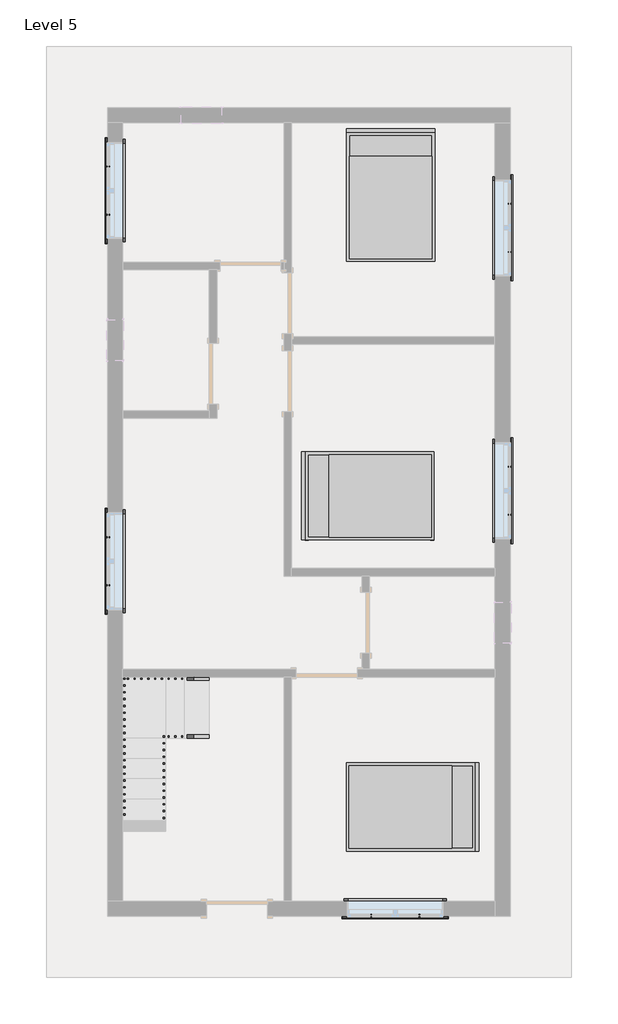
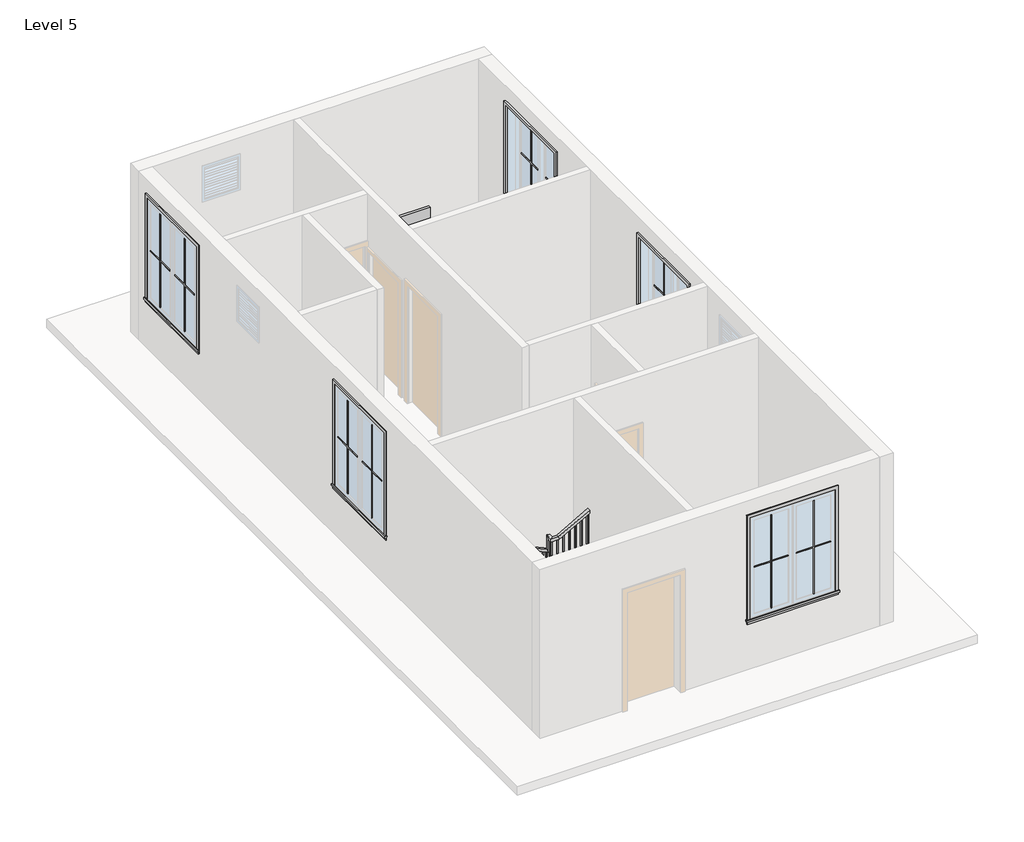
# One storey, part 2 of 2: 20 proxies, 3 furniture elements, 2 railings.
"""IFC4 building model written with IfcOpenShell, lengths in millimetres."""

from ifc_helpers import new_model, si_unit, frame, origin, place, context, project, spatial, polyline, outline, extrude, faceted_brep, transform, mapped, element, save
from components import muntin_pattern_2x2_muntin_pattern_2x2_bff912c5, muntin_pattern_2x2_muntin_pattern_2x2_c2194282, trim_window_exterior_flat_with_sill_e04b3088, trim_window_interior_flat_picture_frame_2a7685fe, bed_17739_bed_17739_15c61121

model = new_model("IFC4")

# Units and contexts
model_context = context("Model", 3, world=origin())
ifc_project = project(units=[si_unit("LENGTHUNIT", "METRE", prefix="MILLI")], contexts=[model_context])

# Site, building, storey
site = spatial("IfcSite", under=ifc_project)
building = spatial("IfcBuilding", under=site)
storey = spatial("IfcBuildingStorey", under=building, Name="Level 5", Elevation=9601.2)

# Proxies
placement = place(None, origin())
muntin_pattern_2x2_muntin_pattern_2x2_shape = muntin_pattern_2x2_muntin_pattern_2x2_bff912c5(model_context)
element("IfcBuildingElementProxy", 1, Name="Muntin Pattern_2x2 : Muntin Pattern_2x2", ObjectType="Muntin Pattern_2x2 : Muntin Pattern_2x2", at=placement, inside=storey, context=model_context, shape_type="MappedRepresentation", body=[
    mapped(muntin_pattern_2x2_muntin_pattern_2x2_shape, transform((-4261.9639285, 4584.2694249, 10585.45), x_axis=(0.0, 1.0, 0.0), y_axis=(-1.0, 0.0, 0.0), z_axis=(0.0, 0.0, 1.0))),
])
element("IfcBuildingElementProxy", 2, Name="Muntin Pattern_2x2 : Muntin Pattern_2x2", ObjectType="Muntin Pattern_2x2 : Muntin Pattern_2x2", at=placement, inside=storey, context=model_context, shape_type="MappedRepresentation", body=[
    mapped(muntin_pattern_2x2_muntin_pattern_2x2_shape, transform((1751.4860715, 4746.1944249, 10585.45), x_axis=(0.0, -1.0, 0.0), y_axis=(1.0, 0.0, 0.0), z_axis=(0.0, 0.0, 1.0))),
])
element("IfcBuildingElementProxy", 3, Name="Muntin Pattern_2x2 : Muntin Pattern_2x2", ObjectType="Muntin Pattern_2x2 : Muntin Pattern_2x2", at=placement, inside=storey, context=model_context, shape_type="MappedRepresentation", body=[
    mapped(muntin_pattern_2x2_muntin_pattern_2x2_shape, transform((-4261.9639285, -962.4555751, 10585.45), x_axis=(0.0, 1.0, 0.0), y_axis=(-1.0, 0.0, 0.0), z_axis=(0.0, 0.0, 1.0))),
])
element("IfcBuildingElementProxy", 4, Name="Muntin Pattern_2x2 : Muntin Pattern_2x2", ObjectType="Muntin Pattern_2x2 : Muntin Pattern_2x2", at=placement, inside=storey, context=model_context, shape_type="MappedRepresentation", body=[
    mapped(muntin_pattern_2x2_muntin_pattern_2x2_shape, transform((1751.4860715, 812.3694249, 10585.45), x_axis=(0.0, -1.0, 0.0), y_axis=(1.0, 0.0, 0.0), z_axis=(0.0, 0.0, 1.0))),
])
element("IfcBuildingElementProxy", 5, Name="Muntin Pattern_2x2 : Muntin Pattern_2x2", ObjectType="Muntin Pattern_2x2 : Muntin Pattern_2x2", at=placement, inside=storey, context=model_context, shape_type="MappedRepresentation", body=[
    mapped(muntin_pattern_2x2_muntin_pattern_2x2_shape, transform((397.3485715, -5907.5180751, 10585.45), x_axis=(-1.0, 0.0, 0.0), y_axis=(0.0, -1.0, 0.0), z_axis=(0.0, 0.0, 1.0))),
])
muntin_pattern_2x2_muntin_pattern_2x2_2_shape = muntin_pattern_2x2_muntin_pattern_2x2_c2194282(model_context)
element("IfcBuildingElementProxy", 6, Name="Muntin Pattern_2x2 : Muntin Pattern_2x2", ObjectType="Muntin Pattern_2x2 : Muntin Pattern_2x2", at=placement, inside=storey, context=model_context, shape_type="MappedRepresentation", body=[
    mapped(muntin_pattern_2x2_muntin_pattern_2x2_2_shape, transform((-4261.9639285, 5304.9944249, 10585.45), x_axis=(0.0, -1.0, 0.0), y_axis=(1.0, 0.0, 0.0), z_axis=(0.0, 0.0, 1.0))),
])
element("IfcBuildingElementProxy", 7, Name="Muntin Pattern_2x2 : Muntin Pattern_2x2", ObjectType="Muntin Pattern_2x2 : Muntin Pattern_2x2", at=placement, inside=storey, context=model_context, shape_type="MappedRepresentation", body=[
    mapped(muntin_pattern_2x2_muntin_pattern_2x2_2_shape, transform((1751.4860715, 4025.4694249, 10585.45), x_axis=(0.0, 1.0, 0.0), y_axis=(-1.0, 0.0, 0.0), z_axis=(0.0, 0.0, 1.0))),
])
element("IfcBuildingElementProxy", 8, Name="Muntin Pattern_2x2 : Muntin Pattern_2x2", ObjectType="Muntin Pattern_2x2 : Muntin Pattern_2x2", at=placement, inside=storey, context=model_context, shape_type="MappedRepresentation", body=[
    mapped(muntin_pattern_2x2_muntin_pattern_2x2_2_shape, transform((-4261.9639285, -241.7305751, 10585.45), x_axis=(0.0, -1.0, 0.0), y_axis=(1.0, 0.0, 0.0), z_axis=(0.0, 0.0, 1.0))),
])
element("IfcBuildingElementProxy", 9, Name="Muntin Pattern_2x2 : Muntin Pattern_2x2", ObjectType="Muntin Pattern_2x2 : Muntin Pattern_2x2", at=placement, inside=storey, context=model_context, shape_type="MappedRepresentation", body=[
    mapped(muntin_pattern_2x2_muntin_pattern_2x2_2_shape, transform((1751.4860715, 91.6444249, 10585.45), x_axis=(0.0, 1.0, 0.0), y_axis=(-1.0, 0.0, 0.0), z_axis=(0.0, 0.0, 1.0))),
])
element("IfcBuildingElementProxy", 10, Name="Muntin Pattern_2x2 : Muntin Pattern_2x2", ObjectType="Muntin Pattern_2x2 : Muntin Pattern_2x2", at=placement, inside=storey, context=model_context, shape_type="MappedRepresentation", body=[
    mapped(muntin_pattern_2x2_muntin_pattern_2x2_2_shape, transform((-323.3764285, -5907.5180751, 10585.45), x_axis=(1.0, 0.0, 0.0), y_axis=(0.0, 1.0, 0.0), z_axis=(0.0, 0.0, 1.0))),
])
trim_window_exterior_flat_with_sill_shape = trim_window_exterior_flat_with_sill_e04b3088(model_context)
element("IfcBuildingElementProxy", 11, Name="Trim-Window-Exterior-Flat : with Sill", ObjectType="Trim-Window-Exterior-Flat : with Sill", at=placement, inside=storey, context=model_context, shape_type="MappedRepresentation", body=[
    mapped(trim_window_exterior_flat_with_sill_shape, transform((-4271.4889285, 4944.6319249, 12344.4), x_axis=(0.0, -1.0, 0.0), y_axis=(0.0, 0.0, 1.0), z_axis=(-1.0, 0.0, 0.0))),
])
element("IfcBuildingElementProxy", 12, Name="Trim-Window-Exterior-Flat : with Sill", ObjectType="Trim-Window-Exterior-Flat : with Sill", at=placement, inside=storey, context=model_context, shape_type="MappedRepresentation", body=[
    mapped(trim_window_exterior_flat_with_sill_shape, transform((1761.0110715, 4385.8319249, 12344.4), x_axis=(0.0, 1.0, 0.0), y_axis=(0.0, 0.0, 1.0), z_axis=(1.0, 0.0, 0.0))),
])
element("IfcBuildingElementProxy", 13, Name="Trim-Window-Exterior-Flat : with Sill", ObjectType="Trim-Window-Exterior-Flat : with Sill", at=placement, inside=storey, context=model_context, shape_type="MappedRepresentation", body=[
    mapped(trim_window_exterior_flat_with_sill_shape, transform((-4271.4889285, -602.0930751, 12344.4), x_axis=(0.0, -1.0, 0.0), y_axis=(0.0, 0.0, 1.0), z_axis=(-1.0, 0.0, 0.0))),
])
element("IfcBuildingElementProxy", 14, Name="Trim-Window-Exterior-Flat : with Sill", ObjectType="Trim-Window-Exterior-Flat : with Sill", at=placement, inside=storey, context=model_context, shape_type="MappedRepresentation", body=[
    mapped(trim_window_exterior_flat_with_sill_shape, transform((1761.0110715, 452.0069249, 12344.4), x_axis=(0.0, 1.0, 0.0), y_axis=(0.0, 0.0, 1.0), z_axis=(1.0, 0.0, 0.0))),
])
element("IfcBuildingElementProxy", 15, Name="Trim-Window-Exterior-Flat : with Sill", ObjectType="Trim-Window-Exterior-Flat : with Sill", at=placement, inside=storey, context=model_context, shape_type="MappedRepresentation", body=[
    mapped(trim_window_exterior_flat_with_sill_shape, transform((36.9860715, -5917.0430751, 12344.4), x_axis=(1.0, 0.0, 0.0), y_axis=(0.0, 0.0, 1.0), z_axis=(0.0, -1.0, 0.0))),
])
trim_window_interior_flat_picture_frame_shape = trim_window_interior_flat_picture_frame_2a7685fe(model_context)
element("IfcBuildingElementProxy", 16, Name="Trim-Window-Interior-Flat : Picture Frame", ObjectType="Trim-Window-Interior-Flat : Picture Frame", at=placement, inside=storey, context=model_context, shape_type="MappedRepresentation", body=[
    mapped(trim_window_interior_flat_picture_frame_shape, transform((-4042.8889285, 4944.6319249, 12344.4), x_axis=(0.0, 1.0, 0.0), y_axis=(0.0, 0.0, 1.0), z_axis=(1.0, 0.0, 0.0))),
])
element("IfcBuildingElementProxy", 17, Name="Trim-Window-Interior-Flat : Picture Frame", ObjectType="Trim-Window-Interior-Flat : Picture Frame", at=placement, inside=storey, context=model_context, shape_type="MappedRepresentation", body=[
    mapped(trim_window_interior_flat_picture_frame_shape, transform((1532.4110715, 4385.8319249, 12344.4), x_axis=(0.0, -1.0, 0.0), y_axis=(0.0, 0.0, 1.0), z_axis=(-1.0, 0.0, 0.0))),
])
element("IfcBuildingElementProxy", 18, Name="Trim-Window-Interior-Flat : Picture Frame", ObjectType="Trim-Window-Interior-Flat : Picture Frame", at=placement, inside=storey, context=model_context, shape_type="MappedRepresentation", body=[
    mapped(trim_window_interior_flat_picture_frame_shape, transform((-4042.8889285, -602.0930751, 12344.4), x_axis=(0.0, 1.0, 0.0), y_axis=(0.0, 0.0, 1.0), z_axis=(1.0, 0.0, 0.0))),
])
element("IfcBuildingElementProxy", 19, Name="Trim-Window-Interior-Flat : Picture Frame", ObjectType="Trim-Window-Interior-Flat : Picture Frame", at=placement, inside=storey, context=model_context, shape_type="MappedRepresentation", body=[
    mapped(trim_window_interior_flat_picture_frame_shape, transform((1532.4110715, 452.0069249, 12344.4), x_axis=(0.0, -1.0, 0.0), y_axis=(0.0, 0.0, 1.0), z_axis=(-1.0, 0.0, 0.0))),
])
element("IfcBuildingElementProxy", 20, Name="Trim-Window-Interior-Flat : Picture Frame", ObjectType="Trim-Window-Interior-Flat : Picture Frame", at=placement, inside=storey, context=model_context, shape_type="MappedRepresentation", body=[
    mapped(trim_window_interior_flat_picture_frame_shape, transform((36.9860715, -5688.4430751, 12344.4), x_axis=(-1.0, 0.0, 0.0), y_axis=(0.0, 0.0, 1.0), z_axis=(0.0, 1.0, 0.0))),
])

# Furniture
bed_17739_bed_17739_shape = bed_17739_bed_17739_15c61121(model_context)
element("IfcFurniture", 21, ObjectType="Bed_17739 : Bed_17739", at=placement, inside=storey, context=model_context, shape_type="MappedRepresentation", body=[
    mapped(bed_17739_bed_17739_shape, transform((-29.6889285, 4852.5569249, 9601.2), x_axis=(1.0, 0.0, 0.0), y_axis=(0.0, 1.0, 0.0), z_axis=(0.0, 0.0, 1.0))),
])
element("IfcFurniture", 22, ObjectType="Bed_17739 : Bed_17739", at=placement, inside=storey, context=model_context, shape_type="MappedRepresentation", body=[
    mapped(bed_17739_bed_17739_shape, transform((-347.1889285, 375.8069249, 9601.2), x_axis=(0.0, 1.0, 0.0), y_axis=(-1.0, 0.0, 0.0), z_axis=(0.0, 0.0, 1.0))),
])
element("IfcFurniture", 23, ObjectType="Bed_17739 : Bed_17739", at=placement, inside=storey, context=model_context, shape_type="MappedRepresentation", body=[
    mapped(bed_17739_bed_17739_shape, transform((275.1110715, -4278.7430751, 9601.2), x_axis=(0.0, -1.0, 0.0), y_axis=(1.0, 0.0, 0.0), z_axis=(0.0, 0.0, 1.0))),
])

# Railings
element("IfcRailing", 24, ObjectType="Handrail - Rectangular", at=placement, inside=storey, context=model_context, shape_type="SolidModel", body=[
    faceted_brep([(-2747.4889285, -2386.4430751, 10684.9333333), (-2747.4889285, -2386.4430751, 10627.7271159), (-2747.4889285, -2335.6430751, 10627.7271159), (-2747.4889285, -2335.6430751, 10684.9333333), (-3396.0267484, -2386.4430751, 11020.7457967), (-3408.3987558, -2386.4430751, 10969.9457967), (-3408.3987558, -2335.6430751, 10969.9457967), (-3396.0267484, -2335.6430751, 11020.7457967), (-3992.0889285, -2386.4430751, 11020.7457967), (-3992.0889285, -2386.4430751, 10969.9457967), (-4042.8889285, -2335.6430751, 10969.9457967), (-4042.8889285, -2335.6430751, 11020.7457967), (-3992.0889285, -2940.1628326, 11020.7457967), (-3992.0889285, -2953.3285634, 10969.9457967), (-4042.8889285, -2953.3285634, 10969.9457967), (-4042.8889285, -2940.1628326, 11020.7457967), (-3992.0889285, -5061.9991591, 12199.7618165), (-3992.0889285, -5075.1648899, 12148.9618165), (-4042.8889285, -5075.1648899, 12148.9618165), (-4042.8889285, -5061.9991591, 12199.7618165), (-3992.0889285, -5637.6430751, 12199.7618165), (-3992.0889285, -5637.6430751, 12148.9618165), (-4042.8889285, -5688.4430751, 12148.9618165), (-4042.8889285, -5688.4430751, 12199.7618165), (-3418.001852, -5637.6430751, 12199.7618165), (-3404.8062484, -5637.6430751, 12148.9618165), (-3404.8062484, -5688.4430751, 12148.9618165), (-3418.001852, -5688.4430751, 12199.7618165), (-2793.6303845, -5637.6430751, 12547.6), (-2793.6303845, -5688.4430751, 12547.6), (-2793.6303845, -5688.4430751, 12489.4487115), (-2793.6303845, -5637.6430751, 12489.4487115)], [[[0, 1, 2, 3]], [[1, 0, 4, 5]], [[2, 1, 5, 6]], [[3, 2, 6, 7]], [[0, 3, 7, 4]], [[5, 4, 8, 9]], [[6, 5, 9, 10]], [[7, 6, 10, 11]], [[4, 7, 11, 8]], [[9, 8, 12, 13]], [[10, 9, 13, 14]], [[11, 10, 14, 15]], [[8, 11, 15, 12]], [[13, 12, 16, 17]], [[14, 13, 17, 18]], [[15, 14, 18, 19]], [[12, 15, 19, 16]], [[17, 16, 20, 21]], [[18, 17, 21, 22]], [[19, 18, 22, 23]], [[16, 19, 23, 20]], [[21, 20, 24, 25]], [[22, 21, 25, 26]], [[23, 22, 26, 27]], [[20, 23, 27, 24]], [[28, 29, 30, 31]], [[25, 24, 28, 31]], [[26, 25, 31, 30]], [[27, 26, 30, 29]], [[24, 27, 29, 28]]]),
    extrude(outline(polyline([(12492.1598207, -2788.7639285), (12481.5470401, -2807.8139285), (11463.8666667, -2807.8139285), (11463.8666667, -2788.7639285), (12492.1598207, -2788.7639285)])), frame((0.0, -5672.5680751, 0.0), z_axis=(0.0, 1.0, 0.0), x_axis=(0.0, 0.0, 1.0)), (0.0, 0.0, 1.0), 19.05),
    extrude(outline(polyline([(12435.5583242, -2890.3639285), (12424.9455436, -2909.4139285), (11463.8666667, -2909.4139285), (11463.8666667, -2890.3639285), (12435.5583242, -2890.3639285)])), frame((0.0, -5672.5680751, 0.0), z_axis=(0.0, 1.0, 0.0), x_axis=(0.0, 0.0, 1.0)), (0.0, 0.0, 1.0), 19.05),
    extrude(outline(polyline([(12378.9568277, -2991.9639285), (12368.3440471, -3011.0139285), (11463.8666667, -3011.0139285), (11463.8666667, -2991.9639285), (12378.9568277, -2991.9639285)])), frame((0.0, -5672.5680751, 0.0), z_axis=(0.0, 1.0, 0.0), x_axis=(0.0, 0.0, 1.0)), (0.0, 0.0, 1.0), 19.05),
    extrude(outline(polyline([(12322.3553312, -3093.5639285), (12311.7425506, -3112.6139285), (11463.8666667, -3112.6139285), (11463.8666667, -3093.5639285), (12322.3553312, -3093.5639285)])), frame((0.0, -5672.5680751, 0.0), z_axis=(0.0, 1.0, 0.0), x_axis=(0.0, 0.0, 1.0)), (0.0, 0.0, 1.0), 19.05),
    extrude(outline(polyline([(12265.7538346, -3195.1639285), (12255.1410541, -3214.2139285), (11294.5333333, -3214.2139285), (11294.5333333, -3195.1639285), (12265.7538346, -3195.1639285)])), frame((0.0, -5672.5680751, 0.0), z_axis=(0.0, 1.0, 0.0), x_axis=(0.0, 0.0, 1.0)), (0.0, 0.0, 1.0), 19.05),
    extrude(outline(polyline([(12209.1523381, -3296.7639285), (12198.5395575, -3315.8139285), (11294.5333333, -3315.8139285), (11294.5333333, -3296.7639285), (12209.1523381, -3296.7639285)])), frame((0.0, -5672.5680751, 0.0), z_axis=(0.0, 1.0, 0.0), x_axis=(0.0, 0.0, 1.0)), (0.0, 0.0, 1.0), 19.05),
    extrude(outline(polyline([(12152.5508416, -3398.3639285), (12141.938061, -3417.4139285), (11125.2, -3417.4139285), (11125.2, -3398.3639285), (12152.5508416, -3398.3639285)])), frame((0.0, -5672.5680751, 0.0), z_axis=(0.0, 1.0, 0.0), x_axis=(0.0, 0.0, 1.0)), (0.0, 0.0, 1.0), 19.05),
    extrude(outline(polyline([(-3519.0139285, -5672.5680751), (-3519.0139285, -5653.5180751), (-3499.9639285, -5653.5180751), (-3499.9639285, -5672.5680751), (-3519.0139285, -5672.5680751)])), frame((0.0, 0.0, 11125.2), z_axis=(0.0, 0.0, 1.0), x_axis=(1.0, 0.0, 0.0)), (0.0, 0.0, 1.0), 1023.7618165),
    extrude(outline(polyline([(-3620.6139285, -5672.5680751), (-3620.6139285, -5653.5180751), (-3601.5639285, -5653.5180751), (-3601.5639285, -5672.5680751), (-3620.6139285, -5672.5680751)])), frame((0.0, 0.0, 11125.2), z_axis=(0.0, 0.0, 1.0), x_axis=(1.0, 0.0, 0.0)), (0.0, 0.0, 1.0), 1023.7618165),
    extrude(outline(polyline([(-3722.2139285, -5672.5680751), (-3722.2139285, -5653.5180751), (-3703.1639285, -5653.5180751), (-3703.1639285, -5672.5680751), (-3722.2139285, -5672.5680751)])), frame((0.0, 0.0, 11125.2), z_axis=(0.0, 0.0, 1.0), x_axis=(1.0, 0.0, 0.0)), (0.0, 0.0, 1.0), 1023.7618165),
    extrude(outline(polyline([(-3823.8139285, -5672.5680751), (-3823.8139285, -5653.5180751), (-3804.7639285, -5653.5180751), (-3804.7639285, -5672.5680751), (-3823.8139285, -5672.5680751)])), frame((0.0, 0.0, 11125.2), z_axis=(0.0, 0.0, 1.0), x_axis=(1.0, 0.0, 0.0)), (0.0, 0.0, 1.0), 1023.7618165),
    extrude(outline(polyline([(-3925.4139285, -5672.5680751), (-3925.4139285, -5653.5180751), (-3906.3639285, -5653.5180751), (-3906.3639285, -5672.5680751), (-3925.4139285, -5672.5680751)])), frame((0.0, 0.0, 11125.2), z_axis=(0.0, 0.0, 1.0), x_axis=(1.0, 0.0, 0.0)), (0.0, 0.0, 1.0), 1023.7618165),
    extrude(outline(polyline([(-4027.0139285, -5602.7180751), (-4007.9639285, -5602.7180751), (-4007.9639285, -5621.7680751), (-4027.0139285, -5621.7680751), (-4027.0139285, -5602.7180751)])), frame((0.0, 0.0, 11125.2), z_axis=(0.0, 0.0, 1.0), x_axis=(1.0, 0.0, 0.0)), (0.0, 0.0, 1.0), 1023.7618165),
    extrude(outline(polyline([(-4027.0139285, -5501.1180751), (-4007.9639285, -5501.1180751), (-4007.9639285, -5520.1680751), (-4027.0139285, -5520.1680751), (-4027.0139285, -5501.1180751)])), frame((0.0, 0.0, 11125.2), z_axis=(0.0, 0.0, 1.0), x_axis=(1.0, 0.0, 0.0)), (0.0, 0.0, 1.0), 1023.7618165),
    extrude(outline(polyline([(-4027.0139285, -5399.5180751), (-4007.9639285, -5399.5180751), (-4007.9639285, -5418.5680751), (-4027.0139285, -5418.5680751), (-4027.0139285, -5399.5180751)])), frame((0.0, 0.0, 11125.2), z_axis=(0.0, 0.0, 1.0), x_axis=(1.0, 0.0, 0.0)), (0.0, 0.0, 1.0), 1023.7618165),
    extrude(outline(polyline([(-4027.0139285, -5297.9180751), (-4007.9639285, -5297.9180751), (-4007.9639285, -5316.9680751), (-4027.0139285, -5316.9680751), (-4027.0139285, -5297.9180751)])), frame((0.0, 0.0, 11125.2), z_axis=(0.0, 0.0, 1.0), x_axis=(1.0, 0.0, 0.0)), (0.0, 0.0, 1.0), 1023.7618165),
    extrude(outline(polyline([(-4027.0139285, -5196.3180751), (-4007.9639285, -5196.3180751), (-4007.9639285, -5215.3680751), (-4027.0139285, -5215.3680751), (-4027.0139285, -5196.3180751)])), frame((0.0, 0.0, 11125.2), z_axis=(0.0, 0.0, 1.0), x_axis=(1.0, 0.0, 0.0)), (0.0, 0.0, 1.0), 1023.7618165),
    extrude(outline(polyline([(-4027.0139285, -5094.7180751), (-4007.9639285, -5094.7180751), (-4007.9639285, -5113.7680751), (-4027.0139285, -5113.7680751), (-4027.0139285, -5094.7180751)])), frame((0.0, 0.0, 11125.2), z_axis=(0.0, 0.0, 1.0), x_axis=(1.0, 0.0, 0.0)), (0.0, 0.0, 1.0), 1023.7618165),
    extrude(outline(polyline([(-5012.1680751, 12113.9571119), (-4993.1180751, 12103.3718208), (-4993.1180751, 11125.2), (-5012.1680751, 11125.2), (-5012.1680751, 12113.9571119)])), frame((-4027.0139285, 0.0, 0.0), z_axis=(1.0, 0.0, 0.0), x_axis=(0.0, 1.0, 0.0)), (0.0, 0.0, 1.0), 19.05),
    extrude(outline(polyline([(-4910.5680751, 12057.5022261), (-4891.5180751, 12046.916935), (-4891.5180751, 11125.2), (-4910.5680751, 11125.2), (-4910.5680751, 12057.5022261)])), frame((-4027.0139285, 0.0, 0.0), z_axis=(1.0, 0.0, 0.0), x_axis=(0.0, 1.0, 0.0)), (0.0, 0.0, 1.0), 19.05),
    extrude(outline(polyline([(-4808.9680751, 12001.0473402), (-4789.9180751, 11990.4620491), (-4789.9180751, 11125.2), (-4808.9680751, 11125.2), (-4808.9680751, 12001.0473402)])), frame((-4027.0139285, 0.0, 0.0), z_axis=(1.0, 0.0, 0.0), x_axis=(0.0, 1.0, 0.0)), (0.0, 0.0, 1.0), 19.05),
    extrude(outline(polyline([(-4707.3680751, 11944.4358332), (-4688.3180751, 11933.8505421), (-4688.3180751, 10955.8666667), (-4707.3680751, 10955.8666667), (-4707.3680751, 11944.4358332)])), frame((-4027.0139285, 0.0, 0.0), z_axis=(1.0, 0.0, 0.0), x_axis=(0.0, 1.0, 0.0)), (0.0, 0.0, 1.0), 19.05),
    extrude(outline(polyline([(-4605.7680751, 11887.9809474), (-4586.7180751, 11877.3956563), (-4586.7180751, 10955.8666667), (-4605.7680751, 10955.8666667), (-4605.7680751, 11887.9809474)])), frame((-4027.0139285, 0.0, 0.0), z_axis=(1.0, 0.0, 0.0), x_axis=(0.0, 1.0, 0.0)), (0.0, 0.0, 1.0), 19.05),
    extrude(outline(polyline([(-4504.1680751, 11831.5260615), (-4485.1180751, 11820.9407704), (-4485.1180751, 10955.8666667), (-4504.1680751, 10955.8666667), (-4504.1680751, 11831.5260615)])), frame((-4027.0139285, 0.0, 0.0), z_axis=(1.0, 0.0, 0.0), x_axis=(0.0, 1.0, 0.0)), (0.0, 0.0, 1.0), 19.05),
    extrude(outline(polyline([(-4402.5680751, 11775.1024999), (-4383.5180751, 11764.5172088), (-4383.5180751, 10786.5333333), (-4402.5680751, 10786.5333333), (-4402.5680751, 11775.1024999)])), frame((-4027.0139285, 0.0, 0.0), z_axis=(1.0, 0.0, 0.0), x_axis=(0.0, 1.0, 0.0)), (0.0, 0.0, 1.0), 19.05),
    extrude(outline(polyline([(-4300.9680751, 11718.647614), (-4281.9180751, 11708.0623229), (-4281.9180751, 10786.5333333), (-4300.9680751, 10786.5333333), (-4300.9680751, 11718.647614)])), frame((-4027.0139285, 0.0, 0.0), z_axis=(1.0, 0.0, 0.0), x_axis=(0.0, 1.0, 0.0)), (0.0, 0.0, 1.0), 19.05),
    extrude(outline(polyline([(-4199.3680751, 11662.1927282), (-4180.3180751, 11651.6074371), (-4180.3180751, 10786.5333333), (-4199.3680751, 10786.5333333), (-4199.3680751, 11662.1927282)])), frame((-4027.0139285, 0.0, 0.0), z_axis=(1.0, 0.0, 0.0), x_axis=(0.0, 1.0, 0.0)), (0.0, 0.0, 1.0), 19.05),
    extrude(outline(polyline([(-4097.7680751, 11605.7691666), (-4078.7180751, 11595.1838755), (-4078.7180751, 10617.2), (-4097.7680751, 10617.2), (-4097.7680751, 11605.7691666)])), frame((-4027.0139285, 0.0, 0.0), z_axis=(1.0, 0.0, 0.0), x_axis=(0.0, 1.0, 0.0)), (0.0, 0.0, 1.0), 19.05),
    extrude(outline(polyline([(-3996.1680751, 11549.3142807), (-3977.1180751, 11538.7289896), (-3977.1180751, 10617.2), (-3996.1680751, 10617.2), (-3996.1680751, 11549.3142807)])), frame((-4027.0139285, 0.0, 0.0), z_axis=(1.0, 0.0, 0.0), x_axis=(0.0, 1.0, 0.0)), (0.0, 0.0, 1.0), 19.05),
    extrude(outline(polyline([(-3894.5680751, 11492.8593949), (-3875.5180751, 11482.2741038), (-3875.5180751, 10617.2), (-3894.5680751, 10617.2), (-3894.5680751, 11492.8593949)])), frame((-4027.0139285, 0.0, 0.0), z_axis=(1.0, 0.0, 0.0), x_axis=(0.0, 1.0, 0.0)), (0.0, 0.0, 1.0), 19.05),
    extrude(outline(polyline([(-3792.9680751, 11436.4358332), (-3773.9180751, 11425.8505421), (-3773.9180751, 10447.8666667), (-3792.9680751, 10447.8666667), (-3792.9680751, 11436.4358332)])), frame((-4027.0139285, 0.0, 0.0), z_axis=(1.0, 0.0, 0.0), x_axis=(0.0, 1.0, 0.0)), (0.0, 0.0, 1.0), 19.05),
    extrude(outline(polyline([(-3691.3680751, 11379.9809474), (-3672.3180751, 11369.3956563), (-3672.3180751, 10447.8666667), (-3691.3680751, 10447.8666667), (-3691.3680751, 11379.9809474)])), frame((-4027.0139285, 0.0, 0.0), z_axis=(1.0, 0.0, 0.0), x_axis=(0.0, 1.0, 0.0)), (0.0, 0.0, 1.0), 19.05),
    extrude(outline(polyline([(-3589.7680751, 11323.5260615), (-3570.7180751, 11312.9407704), (-3570.7180751, 10447.8666667), (-3589.7680751, 10447.8666667), (-3589.7680751, 11323.5260615)])), frame((-4027.0139285, 0.0, 0.0), z_axis=(1.0, 0.0, 0.0), x_axis=(0.0, 1.0, 0.0)), (0.0, 0.0, 1.0), 19.05),
    extrude(outline(polyline([(-3488.1680751, 11267.1024999), (-3469.1180751, 11256.5172088), (-3469.1180751, 10278.5333333), (-3488.1680751, 10278.5333333), (-3488.1680751, 11267.1024999)])), frame((-4027.0139285, 0.0, 0.0), z_axis=(1.0, 0.0, 0.0), x_axis=(0.0, 1.0, 0.0)), (0.0, 0.0, 1.0), 19.05),
    extrude(outline(polyline([(-3386.5680751, 11210.647614), (-3367.5180751, 11200.0623229), (-3367.5180751, 10278.5333333), (-3386.5680751, 10278.5333333), (-3386.5680751, 11210.647614)])), frame((-4027.0139285, 0.0, 0.0), z_axis=(1.0, 0.0, 0.0), x_axis=(0.0, 1.0, 0.0)), (0.0, 0.0, 1.0), 19.05),
    extrude(outline(polyline([(-3284.9680751, 11154.1927282), (-3265.9180751, 11143.6074371), (-3265.9180751, 10278.5333333), (-3284.9680751, 10278.5333333), (-3284.9680751, 11154.1927282)])), frame((-4027.0139285, 0.0, 0.0), z_axis=(1.0, 0.0, 0.0), x_axis=(0.0, 1.0, 0.0)), (0.0, 0.0, 1.0), 19.05),
    extrude(outline(polyline([(-3183.3680751, 11097.7691666), (-3164.3180751, 11087.1838755), (-3164.3180751, 10109.2), (-3183.3680751, 10109.2), (-3183.3680751, 11097.7691666)])), frame((-4027.0139285, 0.0, 0.0), z_axis=(1.0, 0.0, 0.0), x_axis=(0.0, 1.0, 0.0)), (0.0, 0.0, 1.0), 19.05),
    extrude(outline(polyline([(-3081.7680751, 11041.3142807), (-3062.7180751, 11030.7289896), (-3062.7180751, 10109.2), (-3081.7680751, 10109.2), (-3081.7680751, 11041.3142807)])), frame((-4027.0139285, 0.0, 0.0), z_axis=(1.0, 0.0, 0.0), x_axis=(0.0, 1.0, 0.0)), (0.0, 0.0, 1.0), 19.05),
    extrude(outline(polyline([(-2980.1680751, 10984.8593949), (-2961.1180751, 10974.2741038), (-2961.1180751, 10109.2), (-2980.1680751, 10109.2), (-2980.1680751, 10984.8593949)])), frame((-4027.0139285, 0.0, 0.0), z_axis=(1.0, 0.0, 0.0), x_axis=(0.0, 1.0, 0.0)), (0.0, 0.0, 1.0), 19.05),
    extrude(outline(polyline([(-4027.0139285, -2859.5180751), (-4007.9639285, -2859.5180751), (-4007.9639285, -2878.5680751), (-4027.0139285, -2878.5680751), (-4027.0139285, -2859.5180751)])), frame((0.0, 0.0, 10109.2), z_axis=(0.0, 0.0, 1.0), x_axis=(1.0, 0.0, 0.0)), (0.0, 0.0, 1.0), 860.7457967),
    extrude(outline(polyline([(-4027.0139285, -2757.9180751), (-4007.9639285, -2757.9180751), (-4007.9639285, -2776.9680751), (-4027.0139285, -2776.9680751), (-4027.0139285, -2757.9180751)])), frame((0.0, 0.0, 10109.2), z_axis=(0.0, 0.0, 1.0), x_axis=(1.0, 0.0, 0.0)), (0.0, 0.0, 1.0), 860.7457967),
    extrude(outline(polyline([(-4027.0139285, -2656.3180751), (-4007.9639285, -2656.3180751), (-4007.9639285, -2675.3680751), (-4027.0139285, -2675.3680751), (-4027.0139285, -2656.3180751)])), frame((0.0, 0.0, 10109.2), z_axis=(0.0, 0.0, 1.0), x_axis=(1.0, 0.0, 0.0)), (0.0, 0.0, 1.0), 860.7457967),
    extrude(outline(polyline([(-4027.0139285, -2554.7180751), (-4007.9639285, -2554.7180751), (-4007.9639285, -2573.7680751), (-4027.0139285, -2573.7680751), (-4027.0139285, -2554.7180751)])), frame((0.0, 0.0, 10109.2), z_axis=(0.0, 0.0, 1.0), x_axis=(1.0, 0.0, 0.0)), (0.0, 0.0, 1.0), 860.7457967),
    extrude(outline(polyline([(-4027.0139285, -2453.1180751), (-4007.9639285, -2453.1180751), (-4007.9639285, -2472.1680751), (-4027.0139285, -2472.1680751), (-4027.0139285, -2453.1180751)])), frame((0.0, 0.0, 10109.2), z_axis=(0.0, 0.0, 1.0), x_axis=(1.0, 0.0, 0.0)), (0.0, 0.0, 1.0), 860.7457967),
    extrude(outline(polyline([(-3957.1639285, -2351.5180751), (-3957.1639285, -2370.5680751), (-3976.2139285, -2370.5680751), (-3976.2139285, -2351.5180751), (-3957.1639285, -2351.5180751)])), frame((0.0, 0.0, 10109.2), z_axis=(0.0, 0.0, 1.0), x_axis=(1.0, 0.0, 0.0)), (0.0, 0.0, 1.0), 860.7457967),
    extrude(outline(polyline([(-3855.5639285, -2351.5180751), (-3855.5639285, -2370.5680751), (-3874.6139285, -2370.5680751), (-3874.6139285, -2351.5180751), (-3855.5639285, -2351.5180751)])), frame((0.0, 0.0, 10109.2), z_axis=(0.0, 0.0, 1.0), x_axis=(1.0, 0.0, 0.0)), (0.0, 0.0, 1.0), 860.7457967),
    extrude(outline(polyline([(-3753.9639285, -2351.5180751), (-3753.9639285, -2370.5680751), (-3773.0139285, -2370.5680751), (-3773.0139285, -2351.5180751), (-3753.9639285, -2351.5180751)])), frame((0.0, 0.0, 10109.2), z_axis=(0.0, 0.0, 1.0), x_axis=(1.0, 0.0, 0.0)), (0.0, 0.0, 1.0), 860.7457967),
    extrude(outline(polyline([(-3652.3639285, -2351.5180751), (-3652.3639285, -2370.5680751), (-3671.4139285, -2370.5680751), (-3671.4139285, -2351.5180751), (-3652.3639285, -2351.5180751)])), frame((0.0, 0.0, 10109.2), z_axis=(0.0, 0.0, 1.0), x_axis=(1.0, 0.0, 0.0)), (0.0, 0.0, 1.0), 860.7457967),
    extrude(outline(polyline([(-3550.7639285, -2351.5180751), (-3550.7639285, -2370.5680751), (-3569.8139285, -2370.5680751), (-3569.8139285, -2351.5180751), (-3550.7639285, -2351.5180751)])), frame((0.0, 0.0, 10109.2), z_axis=(0.0, 0.0, 1.0), x_axis=(1.0, 0.0, 0.0)), (0.0, 0.0, 1.0), 860.7457967),
    extrude(outline(polyline([(-3449.1639285, -2351.5180751), (-3449.1639285, -2370.5680751), (-3468.2139285, -2370.5680751), (-3468.2139285, -2351.5180751), (-3449.1639285, -2351.5180751)])), frame((0.0, 0.0, 10109.2), z_axis=(0.0, 0.0, 1.0), x_axis=(1.0, 0.0, 0.0)), (0.0, 0.0, 1.0), 860.7457967),
    extrude(outline(polyline([(10938.4455625, -3347.5639285), (10948.3096402, -3366.6139285), (9939.8666667, -3366.6139285), (9939.8666667, -3347.5639285), (10938.4455625, -3347.5639285)])), frame((0.0, -2370.5680751, 0.0), z_axis=(0.0, 1.0, 0.0), x_axis=(0.0, 0.0, 1.0)), (0.0, 0.0, 1.0), 19.05),
    extrude(outline(polyline([(10885.8371483, -3245.9639285), (10895.7012259, -3265.0139285), (9939.8666667, -3265.0139285), (9939.8666667, -3245.9639285), (10885.8371483, -3245.9639285)])), frame((0.0, -2370.5680751, 0.0), z_axis=(0.0, 1.0, 0.0), x_axis=(0.0, 0.0, 1.0)), (0.0, 0.0, 1.0), 19.05),
    extrude(outline(polyline([(10833.228734, -3144.3639285), (10843.0928117, -3163.4139285), (9939.8666667, -3163.4139285), (9939.8666667, -3144.3639285), (10833.228734, -3144.3639285)])), frame((0.0, -2370.5680751, 0.0), z_axis=(0.0, 1.0, 0.0), x_axis=(0.0, 0.0, 1.0)), (0.0, 0.0, 1.0), 19.05),
    extrude(outline(polyline([(10780.6203198, -3042.7639285), (10790.4843975, -3061.8139285), (9770.5333333, -3061.8139285), (9770.5333333, -3042.7639285), (10780.6203198, -3042.7639285)])), frame((0.0, -2370.5680751, 0.0), z_axis=(0.0, 1.0, 0.0), x_axis=(0.0, 0.0, 1.0)), (0.0, 0.0, 1.0), 19.05),
    extrude(outline(polyline([(10728.0119056, -2941.1639285), (10737.8759832, -2960.2139285), (9770.5333333, -2960.2139285), (9770.5333333, -2941.1639285), (10728.0119056, -2941.1639285)])), frame((0.0, -2370.5680751, 0.0), z_axis=(0.0, 1.0, 0.0), x_axis=(0.0, 0.0, 1.0)), (0.0, 0.0, 1.0), 19.05),
    extrude(outline(polyline([(10675.4034913, -2839.5639285), (10685.267569, -2858.6139285), (9770.5333333, -2858.6139285), (9770.5333333, -2839.5639285), (10675.4034913, -2839.5639285)])), frame((0.0, -2370.5680751, 0.0), z_axis=(0.0, 1.0, 0.0), x_axis=(0.0, 0.0, 1.0)), (0.0, 0.0, 1.0), 19.05),
    extrude(outline(polyline([(-4027.0139285, -5653.5180751), (-4007.9639285, -5653.5180751), (-4007.9639285, -5672.5680751), (-4027.0139285, -5672.5680751), (-4027.0139285, -5653.5180751)])), frame((0.0, 0.0, 11125.2), z_axis=(0.0, 0.0, 1.0), x_axis=(1.0, 0.0, 0.0)), (0.0, 0.0, 1.0), 1023.7618165),
    extrude(outline(polyline([(-4007.9639285, -2351.5180751), (-4007.9639285, -2370.5680751), (-4027.0139285, -2370.5680751), (-4027.0139285, -2351.5180751), (-4007.9639285, -2351.5180751)])), frame((0.0, 0.0, 10109.2), z_axis=(0.0, 0.0, 1.0), x_axis=(1.0, 0.0, 0.0)), (0.0, 0.0, 1.0), 860.7457967),
    extrude(outline(polyline([(12489.4487115, -2793.6303845), (12478.8359309, -2812.6803845), (11463.8666667, -2812.6803845), (11463.8666667, -2793.6303845), (12489.4487115, -2793.6303845)])), frame((0.0, -5672.5680751, 0.0), z_axis=(0.0, 1.0, 0.0), x_axis=(0.0, 0.0, 1.0)), (0.0, 0.0, 1.0), 19.05),
    extrude(outline(polyline([(10627.7271159, -2747.4889285), (10637.5911936, -2766.5389285), (9770.5333333, -2766.5389285), (9770.5333333, -2747.4889285), (10627.7271159, -2747.4889285)])), frame((0.0, -2370.5680751, 0.0), z_axis=(0.0, 1.0, 0.0), x_axis=(0.0, 0.0, 1.0)), (0.0, 0.0, 1.0), 19.05),
])
element("IfcRailing", 25, ObjectType="Handrail - Rectangular", at=placement, inside=storey, context=model_context, shape_type="SolidModel", body=[
    faceted_brep([(-2747.4889285, -3250.0430751, 10684.9333333), (-2747.4889285, -3250.0430751, 10627.7271159), (-2747.4889285, -3199.2430751, 10627.7271159), (-2747.4889285, -3199.2430751, 10684.9333333), (-3325.3389285, -3250.0430751, 10984.1436893), (-3376.1389285, -3250.0430751, 10953.241679), (-3376.1389285, -3199.2430751, 10953.241679), (-3325.3389285, -3199.2430751, 10984.1436893), (-3325.3389285, -3250.0430751, 11235.2744977), (-3376.1389285, -3250.0430751, 11184.4744977), (-3376.1389285, -3199.2430751, 11184.4744977), (-3325.3389285, -3199.2430751, 11235.2744977), (-3401.5389285, -3250.0430751, 11235.2744977), (-3401.5389285, -3250.0430751, 11184.4744977), (-3452.3389285, -3199.2430751, 11184.4744977), (-3452.3389285, -3199.2430751, 11235.2744977), (-3401.5389285, -3326.2430751, 11235.2744977), (-3401.5389285, -3339.4088059, 11184.4744977), (-3452.3389285, -3339.4088059, 11184.4744977), (-3452.3389285, -3326.2430751, 11235.2744977), (-3401.5389285, -4697.5612092, 11997.2588356), (-3401.5389285, -4748.3612092, 11967.3706306), (-3452.3389285, -4748.3612092, 11967.3706306), (-3452.3389285, -4697.5612092, 11997.2588356), (-3401.5389285, -4697.5612092, 12251.3844557), (-3401.5389285, -4748.3612092, 12200.5844557), (-3452.3389285, -4748.3612092, 12200.5844557), (-3452.3389285, -4697.5612092, 12251.3844557), (-3401.5389285, -4773.7612092, 12251.3844557), (-3401.5389285, -4773.7612092, 12200.5844557), (-3452.3389285, -4824.5612092, 12200.5844557), (-3452.3389285, -4824.5612092, 12251.3844557), (-3325.3389285, -4773.7612092, 12251.3844557), (-3312.1433249, -4773.7612092, 12200.5844557), (-3312.1433249, -4824.5612092, 12200.5844557), (-3325.3389285, -4824.5612092, 12251.3844557), (-2793.6303845, -4773.7612092, 12547.6), (-2793.6303845, -4824.5612092, 12547.6), (-2793.6303845, -4824.5612092, 12489.4487115), (-2793.6303845, -4773.7612092, 12489.4487115)], [[[0, 1, 2, 3]], [[1, 0, 4, 5]], [[2, 1, 5, 6]], [[3, 2, 6, 7]], [[0, 3, 7, 4]], [[5, 4, 8, 9]], [[6, 5, 9, 10]], [[7, 6, 10, 11]], [[4, 7, 11, 8]], [[9, 8, 12, 13]], [[10, 9, 13, 14]], [[11, 10, 14, 15]], [[8, 11, 15, 12]], [[13, 12, 16, 17]], [[14, 13, 17, 18]], [[15, 14, 18, 19]], [[12, 15, 19, 16]], [[17, 16, 20, 21]], [[18, 17, 21, 22]], [[19, 18, 22, 23]], [[16, 19, 23, 20]], [[21, 20, 24, 25]], [[22, 21, 25, 26]], [[23, 22, 26, 27]], [[20, 23, 27, 24]], [[25, 24, 28, 29]], [[26, 25, 29, 30]], [[27, 26, 30, 31]], [[24, 27, 31, 28]], [[29, 28, 32, 33]], [[30, 29, 33, 34]], [[31, 30, 34, 35]], [[28, 31, 35, 32]], [[36, 37, 38, 39]], [[33, 32, 36, 39]], [[34, 33, 39, 38]], [[35, 34, 38, 37]], [[32, 35, 37, 36]]]),
    extrude(outline(polyline([(12470.9342595, -2826.8639285), (11463.8666667, -2826.8639285), (11463.8666667, -2807.8139285), (12481.5470401, -2807.8139285), (12470.9342595, -2826.8639285)])), frame((0.0, -4808.6862092, 0.0), z_axis=(0.0, 1.0, 0.0), x_axis=(0.0, 0.0, 1.0)), (0.0, 0.0, 1.0), 19.05),
    extrude(outline(polyline([(12414.332763, -2928.4639285), (11463.8666667, -2928.4639285), (11463.8666667, -2909.4139285), (12424.9455436, -2909.4139285), (12414.332763, -2928.4639285)])), frame((0.0, -4808.6862092, 0.0), z_axis=(0.0, 1.0, 0.0), x_axis=(0.0, 0.0, 1.0)), (0.0, 0.0, 1.0), 19.05),
    extrude(outline(polyline([(12357.7312665, -3030.0639285), (11463.8666667, -3030.0639285), (11463.8666667, -3011.0139285), (12368.3440471, -3011.0139285), (12357.7312665, -3030.0639285)])), frame((0.0, -4808.6862092, 0.0), z_axis=(0.0, 1.0, 0.0), x_axis=(0.0, 0.0, 1.0)), (0.0, 0.0, 1.0), 19.05),
    extrude(outline(polyline([(12301.12977, -3131.6639285), (11463.8666667, -3131.6639285), (11463.8666667, -3112.6139285), (12311.7425506, -3112.6139285), (12301.12977, -3131.6639285)])), frame((0.0, -4808.6862092, 0.0), z_axis=(0.0, 1.0, 0.0), x_axis=(0.0, 0.0, 1.0)), (0.0, 0.0, 1.0), 19.05),
    extrude(outline(polyline([(12244.5282735, -3233.2639285), (11294.5333333, -3233.2639285), (11294.5333333, -3214.2139285), (12255.1410541, -3214.2139285), (12244.5282735, -3233.2639285)])), frame((0.0, -4808.6862092, 0.0), z_axis=(0.0, 1.0, 0.0), x_axis=(0.0, 0.0, 1.0)), (0.0, 0.0, 1.0), 19.05),
    extrude(outline(polyline([(12187.8662042, -3334.8639285), (11294.5333333, -3334.8639285), (11294.5333333, -3315.8139285), (12198.4514953, -3315.8139285), (12187.8662042, -3334.8639285)])), frame((0.0, -4808.6862092, 0.0), z_axis=(0.0, 1.0, 0.0), x_axis=(0.0, 0.0, 1.0)), (0.0, 0.0, 1.0), 19.05),
    extrude(outline(polyline([(-3417.4139285, -4739.1180751), (-3417.4139285, -4758.1680751), (-3436.4639285, -4758.1680751), (-3436.4639285, -4739.1180751), (-3417.4139285, -4739.1180751)])), frame((0.0, 0.0, 10955.8666667), z_axis=(0.0, 0.0, 1.0), x_axis=(1.0, 0.0, 0.0)), (0.0, 0.0, 1.0), 1244.7177891),
    extrude(outline(polyline([(-4637.5180751, 11905.6544234), (-4637.5180751, 10955.8666667), (-4656.5680751, 10955.8666667), (-4656.5680751, 11916.2397145), (-4637.5180751, 11905.6544234)])), frame((-3436.4639285, 0.0, 0.0), z_axis=(1.0, 0.0, 0.0), x_axis=(0.0, 1.0, 0.0)), (0.0, 0.0, 1.0), 19.05),
    extrude(outline(polyline([(-4535.9180751, 11849.1995376), (-4535.9180751, 10955.8666667), (-4554.9680751, 10955.8666667), (-4554.9680751, 11859.7848287), (-4535.9180751, 11849.1995376)])), frame((-3436.4639285, 0.0, 0.0), z_axis=(1.0, 0.0, 0.0), x_axis=(0.0, 1.0, 0.0)), (0.0, 0.0, 1.0), 19.05),
    extrude(outline(polyline([(-4434.3180751, 11792.775976), (-4434.3180751, 10786.5333333), (-4453.3680751, 10786.5333333), (-4453.3680751, 11803.361267), (-4434.3180751, 11792.775976)])), frame((-3436.4639285, 0.0, 0.0), z_axis=(1.0, 0.0, 0.0), x_axis=(0.0, 1.0, 0.0)), (0.0, 0.0, 1.0), 19.05),
    extrude(outline(polyline([(-4332.7180751, 11736.3210901), (-4332.7180751, 10786.5333333), (-4351.7680751, 10786.5333333), (-4351.7680751, 11746.9063812), (-4332.7180751, 11736.3210901)])), frame((-3436.4639285, 0.0, 0.0), z_axis=(1.0, 0.0, 0.0), x_axis=(0.0, 1.0, 0.0)), (0.0, 0.0, 1.0), 19.05),
    extrude(outline(polyline([(-4231.1180751, 11679.8662042), (-4231.1180751, 10786.5333333), (-4250.1680751, 10786.5333333), (-4250.1680751, 11690.4514953), (-4231.1180751, 11679.8662042)])), frame((-3436.4639285, 0.0, 0.0), z_axis=(1.0, 0.0, 0.0), x_axis=(0.0, 1.0, 0.0)), (0.0, 0.0, 1.0), 19.05),
    extrude(outline(polyline([(-4129.5180751, 11623.4426426), (-4129.5180751, 10617.2), (-4148.5680751, 10617.2), (-4148.5680751, 11634.0279337), (-4129.5180751, 11623.4426426)])), frame((-3436.4639285, 0.0, 0.0), z_axis=(1.0, 0.0, 0.0), x_axis=(0.0, 1.0, 0.0)), (0.0, 0.0, 1.0), 19.05),
    extrude(outline(polyline([(-4027.9180751, 11566.9877568), (-4027.9180751, 10617.2), (-4046.9680751, 10617.2), (-4046.9680751, 11577.5730479), (-4027.9180751, 11566.9877568)])), frame((-3436.4639285, 0.0, 0.0), z_axis=(1.0, 0.0, 0.0), x_axis=(0.0, 1.0, 0.0)), (0.0, 0.0, 1.0), 19.05),
    extrude(outline(polyline([(-3926.3180751, 11510.5328709), (-3926.3180751, 10617.2), (-3945.3680751, 10617.2), (-3945.3680751, 11521.118162), (-3926.3180751, 11510.5328709)])), frame((-3436.4639285, 0.0, 0.0), z_axis=(1.0, 0.0, 0.0), x_axis=(0.0, 1.0, 0.0)), (0.0, 0.0, 1.0), 19.05),
    extrude(outline(polyline([(-3824.7180751, 11454.1093093), (-3824.7180751, 10447.8666667), (-3843.7680751, 10447.8666667), (-3843.7680751, 11464.6946004), (-3824.7180751, 11454.1093093)])), frame((-3436.4639285, 0.0, 0.0), z_axis=(1.0, 0.0, 0.0), x_axis=(0.0, 1.0, 0.0)), (0.0, 0.0, 1.0), 19.05),
    extrude(outline(polyline([(-3723.1180751, 11397.6544234), (-3723.1180751, 10447.8666667), (-3742.1680751, 10447.8666667), (-3742.1680751, 11408.2397145), (-3723.1180751, 11397.6544234)])), frame((-3436.4639285, 0.0, 0.0), z_axis=(1.0, 0.0, 0.0), x_axis=(0.0, 1.0, 0.0)), (0.0, 0.0, 1.0), 19.05),
    extrude(outline(polyline([(-3621.5180751, 11341.1995376), (-3621.5180751, 10447.8666667), (-3640.5680751, 10447.8666667), (-3640.5680751, 11351.7848287), (-3621.5180751, 11341.1995376)])), frame((-3436.4639285, 0.0, 0.0), z_axis=(1.0, 0.0, 0.0), x_axis=(0.0, 1.0, 0.0)), (0.0, 0.0, 1.0), 19.05),
    extrude(outline(polyline([(-3519.9180751, 11284.775976), (-3519.9180751, 10278.5333333), (-3538.9680751, 10278.5333333), (-3538.9680751, 11295.361267), (-3519.9180751, 11284.775976)])), frame((-3436.4639285, 0.0, 0.0), z_axis=(1.0, 0.0, 0.0), x_axis=(0.0, 1.0, 0.0)), (0.0, 0.0, 1.0), 19.05),
    extrude(outline(polyline([(-3418.3180751, 11228.3210901), (-3418.3180751, 10278.5333333), (-3437.3680751, 10278.5333333), (-3437.3680751, 11238.9063812), (-3418.3180751, 11228.3210901)])), frame((-3436.4639285, 0.0, 0.0), z_axis=(1.0, 0.0, 0.0), x_axis=(0.0, 1.0, 0.0)), (0.0, 0.0, 1.0), 19.05),
    extrude(outline(polyline([(-3316.7180751, 11171.8662042), (-3316.7180751, 10278.5333333), (-3335.7680751, 10278.5333333), (-3335.7680751, 11182.4514953), (-3316.7180751, 11171.8662042)])), frame((-3436.4639285, 0.0, 0.0), z_axis=(1.0, 0.0, 0.0), x_axis=(0.0, 1.0, 0.0)), (0.0, 0.0, 1.0), 19.05),
    extrude(outline(polyline([(-3347.5639285, -3234.1680751), (-3366.6139285, -3234.1680751), (-3366.6139285, -3215.1180751), (-3347.5639285, -3215.1180751), (-3347.5639285, -3234.1680751)])), frame((0.0, 0.0, 9939.8666667), z_axis=(0.0, 0.0, 1.0), x_axis=(1.0, 0.0, 0.0)), (0.0, 0.0, 1.0), 1244.6078311),
    extrude(outline(polyline([(10895.7012259, -3265.0139285), (9939.8666667, -3265.0139285), (9939.8666667, -3245.9639285), (10885.8371483, -3245.9639285), (10895.7012259, -3265.0139285)])), frame((0.0, -3234.1680751, 0.0), z_axis=(0.0, 1.0, 0.0), x_axis=(0.0, 0.0, 1.0)), (0.0, 0.0, 1.0), 19.05),
    extrude(outline(polyline([(10843.0928117, -3163.4139285), (9939.8666667, -3163.4139285), (9939.8666667, -3144.3639285), (10833.228734, -3144.3639285), (10843.0928117, -3163.4139285)])), frame((0.0, -3234.1680751, 0.0), z_axis=(0.0, 1.0, 0.0), x_axis=(0.0, 0.0, 1.0)), (0.0, 0.0, 1.0), 19.05),
    extrude(outline(polyline([(10790.4843975, -3061.8139285), (9770.5333333, -3061.8139285), (9770.5333333, -3042.7639285), (10780.6203198, -3042.7639285), (10790.4843975, -3061.8139285)])), frame((0.0, -3234.1680751, 0.0), z_axis=(0.0, 1.0, 0.0), x_axis=(0.0, 0.0, 1.0)), (0.0, 0.0, 1.0), 19.05),
    extrude(outline(polyline([(10737.8759832, -2960.2139285), (9770.5333333, -2960.2139285), (9770.5333333, -2941.1639285), (10728.0119056, -2941.1639285), (10737.8759832, -2960.2139285)])), frame((0.0, -3234.1680751, 0.0), z_axis=(0.0, 1.0, 0.0), x_axis=(0.0, 0.0, 1.0)), (0.0, 0.0, 1.0), 19.05),
    extrude(outline(polyline([(10685.267569, -2858.6139285), (9770.5333333, -2858.6139285), (9770.5333333, -2839.5639285), (10675.4034913, -2839.5639285), (10685.267569, -2858.6139285)])), frame((0.0, -3234.1680751, 0.0), z_axis=(0.0, 1.0, 0.0), x_axis=(0.0, 0.0, 1.0)), (0.0, 0.0, 1.0), 19.05),
    extrude(outline(polyline([(-3417.4139285, -4789.6362092), (-3417.4139285, -4808.6862092), (-3436.4639285, -4808.6862092), (-3436.4639285, -4789.6362092), (-3417.4139285, -4789.6362092)])), frame((0.0, 0.0, 11125.2), z_axis=(0.0, 0.0, 1.0), x_axis=(1.0, 0.0, 0.0)), (0.0, 0.0, 1.0), 1075.3844557),
    extrude(outline(polyline([(-3417.4139285, -3234.1680751), (-3436.4639285, -3234.1680751), (-3436.4639285, -3215.1180751), (-3417.4139285, -3215.1180751), (-3417.4139285, -3234.1680751)])), frame((0.0, 0.0, 10109.2), z_axis=(0.0, 0.0, 1.0), x_axis=(1.0, 0.0, 0.0)), (0.0, 0.0, 1.0), 1075.2744977),
    extrude(outline(polyline([(12478.8359309, -2812.6803845), (11463.8666667, -2812.6803845), (11463.8666667, -2793.6303845), (12489.4487115, -2793.6303845), (12478.8359309, -2812.6803845)])), frame((0.0, -4808.6862092, 0.0), z_axis=(0.0, 1.0, 0.0), x_axis=(0.0, 0.0, 1.0)), (0.0, 0.0, 1.0), 19.05),
    extrude(outline(polyline([(10637.5911936, -2766.5389285), (9770.5333333, -2766.5389285), (9770.5333333, -2747.4889285), (10627.7271159, -2747.4889285), (10637.5911936, -2766.5389285)])), frame((0.0, -3234.1680751, 0.0), z_axis=(0.0, 1.0, 0.0), x_axis=(0.0, 0.0, 1.0)), (0.0, 0.0, 1.0), 19.05),
])

save(model, "model.ifc")

# Revit data of these elements
# Type "Muntin Pattern_2x2 : Muntin Pattern_2x2"
#   Width [instance default] = 4' - 0"
#   Thickness = 0' - 0 1/2"
#   Height [instance default] = 4' - 0"
#   Distance = 0' - 0 3/4"
#   Interior Material [instance default] = none
#   Exterior Material [instance default] = none
#   Default Elevation = 0
# Type "Trim-Window-Exterior-Flat : with Sill"
#   Trim Width = 0' - 2 1/4"
#   Trim Thickness_Picture Frame = 0' - 1 1/4"
#   Trim Thickness_with Sill = 0' - 0 3/4"
#   Sill Thickness = 0' - 1 1/4"
#   Opening Width [instance default] = 2' - 0"
#   Opening Height [instance default] = 3' - 0"
#   Default Elevation = 4' - 0"
#   Sill = yes
#   Picture Frame = no
#   Trim Material [instance default] = none
# Type "Trim-Window-Interior-Flat : Picture Frame"
#   Trim Thickness_Picture Frame = 0' - 1 1/4"
#   Trim Width = 0' - 2 1/4"
#   Trim Thickness_with Sill = 0' - 0 3/4"
#   Sill Thickness = 0' - 1 1/4"
#   Opening Width [instance default] = 2' - 0"
#   Opening Height [instance default] = 3' - 0"
#   Default Elevation = 4' - 0"
#   Sill = no
#   Picture Frame = yes
#   Trim Material [instance default] = none
# Type "Bed_17739 : Bed_17739"
#   Default Elevation = 0
# Type "Handrail - Rectangular"
#   Assembly Code = "C2010400"
#   built-in parameter 1008612 = 0.0416667 (stored number, unit not read)
#   built-in parameter 1008611 = 0.0416667 (stored number, unit not read)
#   built-in parameter 1008609 = 0.333333 (stored number, unit not read)
#   built-in parameter 1008604 = 0.166667 (stored number, unit not read)
#   built-in parameter 1008603 = 0.166667 (stored number, unit not read)
#   Railing Height = 3' - 0"
#   built-in parameter 1008630 = 2
#   built-in parameter 1008610 = 2
#   built-in parameter 1008618 = Baluster - Square : 3/4"
# Elements 1, 2, 3, 4, 5, 6, 7, 8, 9, 10 (IfcBuildingElementProxy, "Muntin Pattern_2x2 : Muntin Pattern_2x2")
#   Width = 1' - 11 1/8"
#   Height = 5' - 6 1/2"
#   Interior Material = Wood - Stained
#   Exterior Material = Clad - White
#   Phase Created = New Construction
#   Materials on its faces: "Clad - White", "Wood - Stained"
# Elements 11, 12, 13, 14, 15 (IfcBuildingElementProxy, "Trim-Window-Exterior-Flat : with Sill")
#   Opening Width = 4' - 9"
#   Opening Height = 6' - 0"
#   Trim Material = Clad - White
#   Phase Created = New Construction
#   Materials on its faces: "Clad - White"
# Elements 16, 17, 18, 19, 20 (IfcBuildingElementProxy, "Trim-Window-Interior-Flat : Picture Frame")
#   Opening Width = 4' - 9"
#   Opening Height = 6' - 0"
#   Trim Material = Wood - Stained
#   Phase Created = New Construction
#   Materials on its faces: "Wood - Stained"
# Elements 21, 22, 23 (IfcFurniture, "Bed_17739 : Bed_17739")
#   Phase Created = New Construction
#   Materials on its faces: "legs", "sheets", "bed frame", "Blanket"
# Elements 24, 25 (IfcRailing, "Handrail - Rectangular")
#   Phase Created = New Construction
# Materials
#   "Clad - White": class "Wood", colour RGB 242 242 238, transparency 0, Cost = 0
#   "Wood - Stained": class "Wood", colour RGB 224 178 126, transparency 0, Cost = 0
#   "legs": colour RGB 90 73 37, transparency 0, Cost = 0
#   "sheets": colour RGB 200 195 176, transparency 0, Cost = 0
#   "bed frame": colour RGB 90 73 37, transparency 0, Cost = 0
#   "Blanket": class "System", colour RGB 59 0 1, transparency 0, Cost = 0
